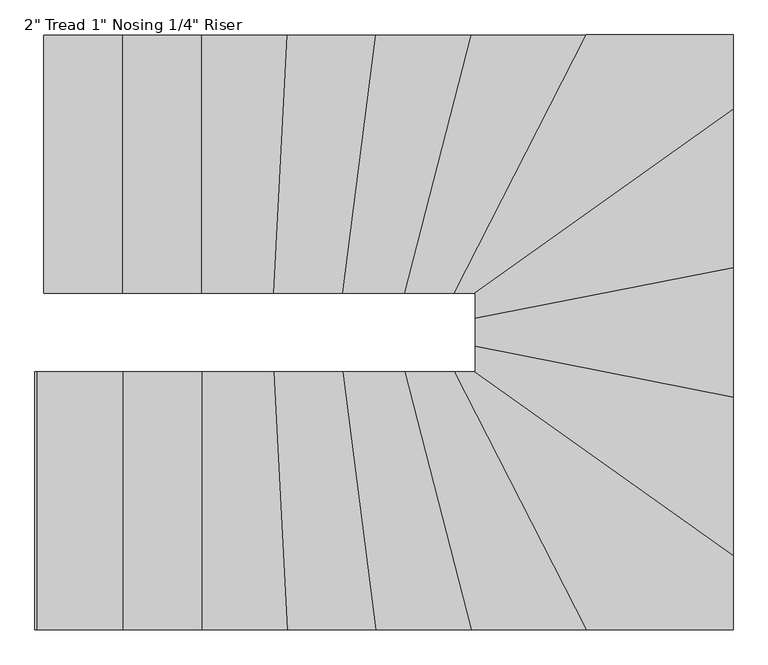
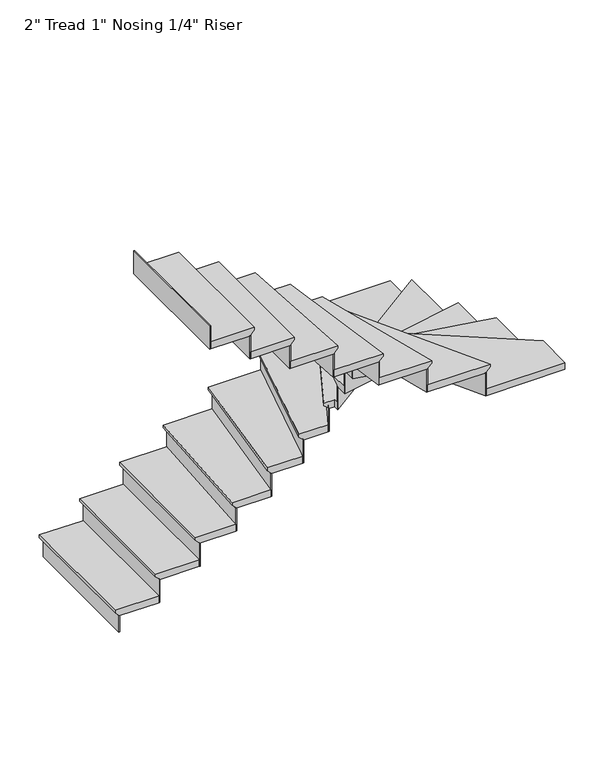
"""IFC4 building model written with IfcOpenShell, lengths in millimetres: stair flight geometry."""

from ifc_helpers import new_model, si_unit, origin, place, context, project, spatial, faceted_brep, source, transform, mapped, element, save


def stair_flight_cc2d1c0a(model_context):
    return source(origin(), model_context, "Body", "Brep", [
        faceted_brep([(3860.8061326, -3914.8192867, 150.2833333), (3860.8061326, -3914.8192867, 169.3333333), (3860.8061326, -3000.4192867, 169.3333333), (3860.8061326, -3000.4192867, 150.2833333), (3886.2061326, -3914.8192867, 124.8833333), (3886.2061326, -3000.4192867, 124.8833333), (4165.6061326, -3914.8192867, 169.3333333), (4165.6061326, -3000.4192867, 169.3333333), (3886.2061326, -3000.4192867, 118.5333333), (4165.6061326, -3000.4192867, 118.5333333), (4165.6061326, -3914.8192867, 118.5333333), (3886.2061326, -3914.8192867, 118.5333333)], [[[0, 1, 2, 3]], [[4, 0, 3, 5]], [[2, 1, 6, 7]], [[8, 9, 10, 11]], [[2, 7, 9, 8, 5, 3]], [[8, 11, 4, 5]], [[6, 1, 0, 4, 11, 10]], [[7, 6, 10, 9]]]),
        faceted_brep([(3886.2061326, -3914.8192867, 118.5333333), (3886.2061326, -3914.8192867, 0.0), (3892.5561326, -3914.8192867, 0.0), (3892.5561326, -3914.8192867, 118.5333333), (3886.2061326, -3000.4192867, 118.5333333), (3892.5561326, -3000.4192867, 118.5333333), (3892.5561326, -3000.4192867, 0.0), (3886.2061326, -3000.4192867, 0.0)], [[[0, 1, 2, 3]], [[4, 5, 6, 7]], [[1, 0, 4, 7]], [[2, 1, 7, 6]], [[3, 2, 6, 5]], [[0, 3, 5, 4]]]),
        faceted_brep([(4165.6061326, -3914.8192867, 287.8666667), (4165.6061326, -3914.8192867, 118.5333333), (4171.9561326, -3914.8192867, 118.5333333), (4171.9561326, -3914.8192867, 287.8666667), (4165.6061326, -3000.4192867, 287.8666667), (4171.9561326, -3000.4192867, 287.8666667), (4171.9561326, -3000.4192867, 118.5333333), (4165.6061326, -3000.4192867, 118.5333333)], [[[0, 1, 2, 3]], [[4, 5, 6, 7]], [[1, 0, 4, 7]], [[2, 1, 7, 6]], [[3, 2, 6, 5]], [[0, 3, 5, 4]]]),
        faceted_brep([(4140.2061326, -3000.4192867, 338.6666667), (4140.2061326, -3914.8192867, 338.6666667), (4445.0061326, -3914.8192867, 338.6666667), (4445.0061326, -3000.4192867, 338.6666667), (4165.6061326, -3000.4192867, 287.8666667), (4445.0061326, -3000.4192867, 287.8666667), (4445.0061326, -3914.8192867, 287.8666667), (4165.6061326, -3914.8192867, 287.8666667), (4165.6061326, -3000.4192867, 294.2166667), (4140.2061326, -3000.4192867, 319.6166667), (4165.6061326, -3914.8192867, 294.2166667), (4140.2061326, -3914.8192867, 319.6166667)], [[[0, 1, 2, 3]], [[4, 5, 6, 7]], [[0, 3, 5, 4, 8, 9]], [[4, 7, 10, 8]], [[2, 1, 11, 10, 7, 6]], [[3, 2, 6, 5]], [[11, 1, 0, 9]], [[10, 11, 9, 8]]]),
        faceted_brep([(4445.0061326, -3914.8192867, 457.2), (4445.0061326, -3914.8192867, 287.8666667), (4451.3561326, -3914.8192867, 287.8666667), (4451.3561326, -3914.8192867, 457.2), (4445.0061326, -3000.4192867, 457.2), (4451.3561326, -3000.4192867, 457.2), (4451.3561326, -3000.4192867, 287.8666667), (4445.0061326, -3000.4192867, 287.8666667)], [[[0, 1, 2, 3]], [[4, 5, 6, 7]], [[1, 0, 4, 7]], [[2, 1, 7, 6]], [[3, 2, 6, 5]], [[0, 3, 5, 4]]]),
        faceted_brep([(4419.6061326, -3000.4192867, 508.0), (4419.6061326, -3914.8192867, 508.0), (4700.6732941, -3914.8192867, 508.0), (4748.2075645, -3000.4192867, 508.0), (4445.0061326, -3000.4192867, 457.2), (4748.2075645, -3000.4192867, 457.2), (4700.6732941, -3914.8192867, 457.2), (4445.0061326, -3914.8192867, 457.2), (4445.0061326, -3000.4192867, 463.55), (4419.6061326, -3000.4192867, 488.95), (4445.0061326, -3914.8192867, 463.55), (4419.6061326, -3914.8192867, 488.95)], [[[0, 1, 2, 3]], [[4, 5, 6, 7]], [[0, 3, 5, 4, 8, 9]], [[4, 7, 10, 8]], [[2, 1, 11, 10, 7, 6]], [[3, 2, 6, 5]], [[11, 1, 0, 9]], [[10, 11, 9, 8]]]),
        faceted_brep([(4700.6732941, -3914.8192867, 626.5333333), (4700.6732941, -3914.8192867, 457.2), (4707.0318682, -3914.8192867, 457.2), (4707.0318682, -3914.8192867, 626.5333333), (4748.2075645, -3000.4192867, 626.5333333), (4754.5661386, -3000.4192867, 626.5333333), (4754.5661386, -3000.4192867, 457.2), (4748.2075645, -3000.4192867, 457.2)], [[[0, 1, 2, 3]], [[4, 5, 6, 7]], [[1, 0, 4, 7]], [[2, 1, 7, 6]], [[3, 2, 6, 5]], [[0, 3, 5, 4]]]),
        faceted_brep([(4722.7732678, -3000.4192867, 677.3333333), (4675.2389974, -3914.8192867, 677.3333333), (4944.8399939, -3914.8192867, 677.3333333), (5063.1960455, -3000.4192867, 677.3333333), (4748.2075645, -3000.4192867, 626.5333333), (5063.1960455, -3000.4192867, 626.5333333), (4944.8399939, -3914.8192867, 626.5333333), (4700.6732941, -3914.8192867, 626.5333333), (4748.2075645, -3000.4192867, 632.8833333), (4722.7732678, -3000.4192867, 658.2833333), (4700.6732941, -3914.8192867, 632.8833333), (4675.2389974, -3914.8192867, 658.2833333)], [[[0, 1, 2, 3]], [[4, 5, 6, 7]], [[0, 3, 5, 4, 8, 9]], [[4, 7, 10, 8]], [[2, 1, 11, 10, 7, 6]], [[3, 2, 6, 5]], [[11, 1, 0, 9]], [[10, 11, 9, 8]]]),
        faceted_brep([(4944.8399939, -3914.8192867, 795.8666667), (4944.8399939, -3914.8192867, 626.5333333), (4951.2429657, -3914.8192867, 626.5333333), (4951.2429657, -3914.8192867, 795.8666667), (5063.1960455, -3000.4192867, 795.8666667), (5069.5990173, -3000.4192867, 795.8666667), (5069.5990173, -3000.4192867, 626.5333333), (5063.1960455, -3000.4192867, 626.5333333)], [[[0, 1, 2, 3]], [[4, 5, 6, 7]], [[1, 0, 4, 7]], [[2, 1, 7, 6]], [[3, 2, 6, 5]], [[0, 3, 5, 4]]]),
        faceted_brep([(5037.5841584, -3000.4192867, 846.6666667), (4919.2281068, -3914.8192867, 846.6666667), (5166.4672164, -3914.8192867, 846.6666667), (5401.5976638, -3000.4192867, 846.6666667), (5063.1960455, -3000.4192867, 795.8666667), (5401.5976638, -3000.4192867, 795.8666667), (5166.4672164, -3914.8192867, 795.8666667), (4944.8399939, -3914.8192867, 795.8666667), (5063.1960455, -3000.4192867, 802.2166667), (5037.5841584, -3000.4192867, 827.6166667), (4944.8399939, -3914.8192867, 802.2166667), (4919.2281068, -3914.8192867, 827.6166667)], [[[0, 1, 2, 3]], [[4, 5, 6, 7]], [[0, 3, 5, 4, 8, 9]], [[4, 7, 10, 8]], [[2, 1, 11, 10, 7, 6]], [[3, 2, 6, 5]], [[11, 1, 0, 9]], [[10, 11, 9, 8]]]),
        faceted_brep([(5166.4672164, -3914.8192867, 965.2), (5166.4672164, -3914.8192867, 795.8666667), (5173.0237932, -3914.8192867, 795.8666667), (5173.0237932, -3914.8192867, 965.2), (5401.5976638, -3000.4192867, 965.2), (5408.1542406, -3000.4192867, 965.2), (5408.1542406, -3000.4192867, 795.8666667), (5401.5976638, -3000.4192867, 795.8666667)], [[[0, 1, 2, 3]], [[4, 5, 6, 7]], [[1, 0, 4, 7]], [[2, 1, 7, 6]], [[3, 2, 6, 5]], [[0, 3, 5, 4]]]),
        faceted_brep([(5375.3713563, -3000.4192867, 1016.0), (5140.2409089, -3914.8192867, 1016.0), (5342.8138524, -3914.8192867, 1016.0), (5811.6384738, -3000.4192867, 1016.0), (5401.5976638, -3000.4192867, 965.2), (5811.6384738, -3000.4192867, 965.2), (5342.8138524, -3914.8192867, 965.2), (5166.4672164, -3914.8192867, 965.2), (5401.5976638, -3000.4192867, 971.55), (5375.3713563, -3000.4192867, 996.95), (5166.4672164, -3914.8192867, 971.55), (5140.2409089, -3914.8192867, 996.95)], [[[0, 1, 2, 3]], [[4, 5, 6, 7]], [[0, 3, 5, 4, 8, 9]], [[4, 7, 10, 8]], [[2, 1, 11, 10, 7, 6]], [[3, 2, 6, 5]], [[11, 1, 0, 9]], [[10, 11, 9, 8]]]),
        faceted_brep([(5342.8138524, -3914.8192867, 1134.5333333), (5342.8138524, -3914.8192867, 965.2), (5349.9498356, -3914.8192867, 965.2), (5349.9498356, -3914.8192867, 1134.5333333), (5811.6384738, -3000.4192867, 1134.5333333), (5818.7744569, -3000.4192867, 1134.5333333), (5818.7744569, -3000.4192867, 965.2), (5811.6384738, -3000.4192867, 965.2)], [[[0, 1, 2, 3]], [[4, 5, 6, 7]], [[1, 0, 4, 7]], [[2, 1, 7, 6]], [[3, 2, 6, 5]], [[0, 3, 5, 4]]]),
        faceted_brep([(6302.9378245, -3294.1004204, 1185.3333333), (6302.9378245, -3000.4192867, 1185.3333333), (5783.0945412, -3000.4192867, 1185.3333333), (5314.2699199, -3914.8192867, 1185.3333333), (5388.5378245, -3914.8192867, 1185.3333333), (5388.5378245, -3944.3743695, 1185.3333333), (6302.9378245, -3000.4192867, 1134.5333333), (6302.9378245, -3294.1004204, 1134.5333333), (5388.5378245, -3944.3743695, 1134.5333333), (5388.5378245, -3914.8192867, 1134.5333333), (5342.8138524, -3914.8192867, 1134.5333333), (5811.6384738, -3000.4192867, 1134.5333333), (5811.6384738, -3000.4192867, 1140.8833333), (5783.0945412, -3000.4192867, 1166.2833333), (5342.8138524, -3914.8192867, 1140.8833333), (5314.2699199, -3914.8192867, 1166.2833333)], [[[0, 1, 2, 3, 4, 5]], [[6, 7, 8, 9, 10, 11]], [[1, 0, 7, 6]], [[2, 1, 6, 11, 12, 13]], [[11, 10, 14, 12]], [[4, 3, 15, 14, 10, 9]], [[5, 4, 9, 8]], [[0, 5, 8, 7]], [[15, 3, 2, 13]], [[14, 15, 13, 12]]]),
        faceted_brep([(5388.5378245, -3944.3743695, 1303.8666667), (5388.5378245, -3944.3743695, 1134.5333333), (5388.5378245, -3952.1663443, 1134.5333333), (5388.5378245, -3952.1663443, 1303.8666667), (6302.9378245, -3294.1004204, 1303.8666667), (6302.9378245, -3301.8923952, 1303.8666667), (6302.9378245, -3301.8923952, 1134.5333333), (6302.9378245, -3294.1004204, 1134.5333333)], [[[0, 1, 2, 3]], [[4, 5, 6, 7]], [[1, 0, 4, 7]], [[2, 1, 7, 6]], [[3, 2, 6, 5]], [[0, 3, 5, 4]]]),
        faceted_brep([(6302.9378245, -3262.9325212, 1354.6666667), (5388.5378245, -3913.2064704, 1354.6666667), (5388.5378245, -4030.8284566, 1354.6666667), (6302.9378245, -3850.5876003, 1354.6666667), (6302.9378245, -3294.1004204, 1303.8666667), (6302.9378245, -3850.5876003, 1303.8666667), (5388.5378245, -4030.8284566, 1303.8666667), (5388.5378245, -3944.3743695, 1303.8666667), (6302.9378245, -3294.1004204, 1310.2166667), (6302.9378245, -3262.9325212, 1335.6166667), (5388.5378245, -3944.3743695, 1310.2166667), (5388.5378245, -3913.2064704, 1335.6166667)], [[[0, 1, 2, 3]], [[4, 5, 6, 7]], [[0, 3, 5, 4, 8, 9]], [[4, 7, 10, 8]], [[2, 1, 11, 10, 7, 6]], [[3, 2, 6, 5]], [[11, 1, 0, 9]], [[10, 11, 9, 8]]]),
        faceted_brep([(5388.5378245, -4030.8284566, 1473.2), (5388.5378245, -4030.8284566, 1303.8666667), (5388.5378245, -4037.300642, 1303.8666667), (5388.5378245, -4037.300642, 1473.2), (6302.9378245, -3850.5876003, 1473.2), (6302.9378245, -3857.0597857, 1473.2), (6302.9378245, -3857.0597857, 1303.8666667), (6302.9378245, -3850.5876003, 1303.8666667)], [[[0, 1, 2, 3]], [[4, 5, 6, 7]], [[1, 0, 4, 7]], [[2, 1, 7, 6]], [[3, 2, 6, 5]], [[0, 3, 5, 4]]]),
        faceted_brep([(6302.9378245, -3824.6988585, 1524.0), (5388.5378245, -4004.9397148, 1524.0), (5388.5378245, -4129.9876003, 1524.0), (6302.9378245, -4310.2284566, 1524.0), (6302.9378245, -3850.5876003, 1473.2), (6302.9378245, -4310.2284566, 1473.2), (5388.5378245, -4129.9876003, 1473.2), (5388.5378245, -4030.8284566, 1473.2), (6302.9378245, -3850.5876003, 1479.55), (6302.9378245, -3824.6988585, 1504.95), (5388.5378245, -4030.8284566, 1479.55), (5388.5378245, -4004.9397148, 1504.95)], [[[0, 1, 2, 3]], [[4, 5, 6, 7]], [[0, 3, 5, 4, 8, 9]], [[4, 7, 10, 8]], [[2, 1, 11, 10, 7, 6]], [[3, 2, 6, 5]], [[11, 1, 0, 9]], [[10, 11, 9, 8]]]),
        faceted_brep([(5388.5378245, -4129.9876003, 1642.5333333), (5388.5378245, -4129.9876003, 1473.2), (5388.5378245, -4136.4597857, 1473.2), (5388.5378245, -4136.4597857, 1642.5333333), (6302.9378245, -4310.2284566, 1642.5333333), (6302.9378245, -4316.700642, 1642.5333333), (6302.9378245, -4316.700642, 1473.2), (6302.9378245, -4310.2284566, 1473.2)], [[[0, 1, 2, 3]], [[4, 5, 6, 7]], [[1, 0, 4, 7]], [[2, 1, 7, 6]], [[3, 2, 6, 5]], [[0, 3, 5, 4]]]),
        faceted_brep([(6302.9378245, -4284.3397148, 1693.3333333), (5388.5378245, -4104.0988585, 1693.3333333), (5388.5378245, -4194.2192867, 1693.3333333), (5342.4423499, -4194.2192867, 1693.3333333), (6302.9378245, -4877.2739513, 1693.3333333), (6302.9378245, -4310.2284566, 1642.5333333), (6302.9378245, -4877.2739513, 1642.5333333), (5342.4423499, -4194.2192867, 1642.5333333), (5388.5378245, -4194.2192867, 1642.5333333), (5388.5378245, -4129.9876003, 1642.5333333), (6302.9378245, -4310.2284566, 1648.8833333), (6302.9378245, -4284.3397148, 1674.2833333), (5388.5378245, -4129.9876003, 1648.8833333), (5388.5378245, -4104.0988585, 1674.2833333)], [[[0, 1, 2, 3, 4]], [[5, 6, 7, 8, 9]], [[0, 4, 6, 5, 10, 11]], [[5, 9, 12, 10]], [[2, 1, 13, 12, 9, 8]], [[3, 2, 8, 7]], [[4, 3, 7, 6]], [[13, 1, 0, 11]], [[12, 13, 11, 10]]]),
        faceted_brep([(5342.4423499, -4194.2192867, 1811.8666667), (5342.4423499, -4194.2192867, 1642.5333333), (5331.4854574, -4194.2192867, 1642.5333333), (5331.4854574, -4194.2192867, 1811.8666667), (6302.9378245, -4877.2739513, 1811.8666667), (6302.9378245, -4885.0659261, 1811.8666667), (6302.9378245, -4885.0659261, 1642.5333333), (6302.9378245, -4877.2739513, 1642.5333333)], [[[0, 1, 2, 3]], [[4, 5, 6, 7]], [[1, 0, 4, 7]], [[2, 1, 7, 6]], [[3, 2, 6, 5]], [[0, 3, 5, 4]]]),
        faceted_brep([(5754.5506087, -5108.6192867, 1862.6666667), (6302.9378245, -5108.6192867, 1862.6666667), (6302.9378245, -4846.1060522, 1862.6666667), (5386.2699199, -4194.2192867, 1862.6666667), (5285.7259874, -4194.2192867, 1862.6666667), (6302.9378245, -5108.6192867, 1811.8666667), (5754.5506087, -5108.6192867, 1811.8666667), (5285.7259874, -4194.2192867, 1811.8666667), (5342.4423499, -4194.2192867, 1811.8666667), (6302.9378245, -4877.2739513, 1811.8666667), (6302.9378245, -4877.2739513, 1818.2166667), (6302.9378245, -4846.1060522, 1843.6166667), (5342.4423499, -4194.2192867, 1818.2166667), (5386.2699199, -4194.2192867, 1843.6166667)], [[[0, 1, 2, 3, 4]], [[5, 6, 7, 8, 9]], [[1, 0, 6, 5]], [[2, 1, 5, 9, 10, 11]], [[9, 8, 12, 10]], [[4, 3, 13, 12, 8, 7]], [[0, 4, 7, 6]], [[13, 3, 2, 11]], [[12, 13, 11, 10]]]),
        faceted_brep([(5285.7259874, -4194.2192867, 1981.2), (5285.7259874, -4194.2192867, 1811.8666667), (5278.5900042, -4194.2192867, 1811.8666667), (5278.5900042, -4194.2192867, 1981.2), (5754.5506087, -5108.6192867, 1981.2), (5747.4146256, -5108.6192867, 1981.2), (5747.4146256, -5108.6192867, 1811.8666667), (5754.5506087, -5108.6192867, 1811.8666667)], [[[0, 1, 2, 3]], [[4, 5, 6, 7]], [[1, 0, 4, 7]], [[2, 1, 7, 6]], [[3, 2, 6, 5]], [[0, 3, 5, 4]]]),
        faceted_brep([(5783.0945412, -5108.6192867, 2032.0), (5314.2699199, -4194.2192867, 2032.0), (5114.0146014, -4194.2192867, 2032.0), (5349.1450488, -5108.6192867, 2032.0), (5754.5506087, -5108.6192867, 1981.2), (5349.1450488, -5108.6192867, 1981.2), (5114.0146014, -4194.2192867, 1981.2), (5285.7259874, -4194.2192867, 1981.2), (5754.5506087, -5108.6192867, 1987.55), (5783.0945412, -5108.6192867, 2012.95), (5285.7259874, -4194.2192867, 1987.55), (5314.2699199, -4194.2192867, 2012.95)], [[[0, 1, 2, 3]], [[4, 5, 6, 7]], [[0, 3, 5, 4, 8, 9]], [[4, 7, 10, 8]], [[2, 1, 11, 10, 7, 6]], [[3, 2, 6, 5]], [[11, 1, 0, 9]], [[10, 11, 9, 8]]]),
        faceted_brep([(5114.0146014, -4194.2192867, 2150.5333333), (5114.0146014, -4194.2192867, 1981.2), (5107.4580246, -4194.2192867, 1981.2), (5107.4580246, -4194.2192867, 2150.5333333), (5349.1450488, -5108.6192867, 2150.5333333), (5342.588472, -5108.6192867, 2150.5333333), (5342.588472, -5108.6192867, 1981.2), (5349.1450488, -5108.6192867, 1981.2)], [[[0, 1, 2, 3]], [[4, 5, 6, 7]], [[1, 0, 4, 7]], [[2, 1, 7, 6]], [[3, 2, 6, 5]], [[0, 3, 5, 4]]]),
        faceted_brep([(5375.3713563, -5108.6192867, 2201.3333333), (5140.2409089, -4194.2192867, 2201.3333333), (4893.6162196, -4194.2192867, 2201.3333333), (5011.9722713, -5108.6192867, 2201.3333333), (5349.1450488, -5108.6192867, 2150.5333333), (5011.9722713, -5108.6192867, 2150.5333333), (4893.6162196, -4194.2192867, 2150.5333333), (5114.0146014, -4194.2192867, 2150.5333333), (5349.1450488, -5108.6192867, 2156.8833333), (5375.3713563, -5108.6192867, 2182.2833333), (5114.0146014, -4194.2192867, 2156.8833333), (5140.2409089, -4194.2192867, 2182.2833333)], [[[0, 1, 2, 3]], [[4, 5, 6, 7]], [[0, 3, 5, 4, 8, 9]], [[4, 7, 10, 8]], [[2, 1, 11, 10, 7, 6]], [[3, 2, 6, 5]], [[11, 1, 0, 9]], [[10, 11, 9, 8]]]),
        faceted_brep([(4893.6162196, -4194.2192867, 2319.8666667), (4893.6162196, -4194.2192867, 2150.5333333), (4887.2132479, -4194.2192867, 2150.5333333), (4887.2132479, -4194.2192867, 2319.8666667), (5011.9722713, -5108.6192867, 2319.8666667), (5005.5692995, -5108.6192867, 2319.8666667), (5005.5692995, -5108.6192867, 2150.5333333), (5011.9722713, -5108.6192867, 2150.5333333)], [[[0, 1, 2, 3]], [[4, 5, 6, 7]], [[1, 0, 4, 7]], [[2, 1, 7, 6]], [[3, 2, 6, 5]], [[0, 3, 5, 4]]]),
        faceted_brep([(5037.5841584, -5108.6192867, 2370.6666667), (4919.2281068, -4194.2192867, 2370.6666667), (4649.8047007, -4194.2192867, 2370.6666667), (4697.3389711, -5108.6192867, 2370.6666667), (5011.9722713, -5108.6192867, 2319.8666667), (4697.3389711, -5108.6192867, 2319.8666667), (4649.8047007, -4194.2192867, 2319.8666667), (4893.6162196, -4194.2192867, 2319.8666667), (5011.9722713, -5108.6192867, 2326.2166667), (5037.5841584, -5108.6192867, 2351.6166667), (4893.6162196, -4194.2192867, 2326.2166667), (4919.2281068, -4194.2192867, 2351.6166667)], [[[0, 1, 2, 3]], [[4, 5, 6, 7]], [[0, 3, 5, 4, 8, 9]], [[4, 7, 10, 8]], [[2, 1, 11, 10, 7, 6]], [[3, 2, 6, 5]], [[11, 1, 0, 9]], [[10, 11, 9, 8]]]),
        faceted_brep([(4649.8047007, -4194.2192867, 2489.2), (4649.8047007, -4194.2192867, 2319.8666667), (4643.4461266, -4194.2192867, 2319.8666667), (4643.4461266, -4194.2192867, 2489.2), (4697.3389711, -5108.6192867, 2489.2), (4690.980397, -5108.6192867, 2489.2), (4690.980397, -5108.6192867, 2319.8666667), (4697.3389711, -5108.6192867, 2319.8666667)], [[[0, 1, 2, 3]], [[4, 5, 6, 7]], [[1, 0, 4, 7]], [[2, 1, 7, 6]], [[3, 2, 6, 5]], [[0, 3, 5, 4]]]),
        faceted_brep([(4722.7732678, -5108.6192867, 2540.0), (4675.2389974, -4194.2192867, 2540.0), (4394.2061326, -4194.2192867, 2540.0), (4394.2061326, -5108.6192867, 2540.0), (4697.3389711, -5108.6192867, 2489.2), (4394.2061326, -5108.6192867, 2489.2), (4394.2061326, -4194.2192867, 2489.2), (4649.8047007, -4194.2192867, 2489.2), (4697.3389711, -5108.6192867, 2495.55), (4722.7732678, -5108.6192867, 2520.95), (4649.8047007, -4194.2192867, 2495.55), (4675.2389974, -4194.2192867, 2520.95)], [[[0, 1, 2, 3]], [[4, 5, 6, 7]], [[0, 3, 5, 4, 8, 9]], [[4, 7, 10, 8]], [[2, 1, 11, 10, 7, 6]], [[3, 2, 6, 5]], [[11, 1, 0, 9]], [[10, 11, 9, 8]]]),
        faceted_brep([(4394.2061326, -4194.2192867, 2658.5333333), (4394.2061326, -4194.2192867, 2489.2), (4387.8561326, -4194.2192867, 2489.2), (4387.8561326, -4194.2192867, 2658.5333333), (4394.2061326, -5108.6192867, 2658.5333333), (4387.8561326, -5108.6192867, 2658.5333333), (4387.8561326, -5108.6192867, 2489.2), (4394.2061326, -5108.6192867, 2489.2)], [[[0, 1, 2, 3]], [[4, 5, 6, 7]], [[1, 0, 4, 7]], [[2, 1, 7, 6]], [[3, 2, 6, 5]], [[0, 3, 5, 4]]]),
        faceted_brep([(4419.6061326, -5108.6192867, 2709.3333333), (4419.6061326, -4194.2192867, 2709.3333333), (4114.8061326, -4194.2192867, 2709.3333333), (4114.8061326, -5108.6192867, 2709.3333333), (4394.2061326, -5108.6192867, 2658.5333333), (4114.8061326, -5108.6192867, 2658.5333333), (4114.8061326, -4194.2192867, 2658.5333333), (4394.2061326, -4194.2192867, 2658.5333333), (4394.2061326, -5108.6192867, 2664.8833333), (4419.6061326, -5108.6192867, 2690.2833333), (4394.2061326, -4194.2192867, 2664.8833333), (4419.6061326, -4194.2192867, 2690.2833333)], [[[0, 1, 2, 3]], [[4, 5, 6, 7]], [[0, 3, 5, 4, 8, 9]], [[4, 7, 10, 8]], [[2, 1, 11, 10, 7, 6]], [[3, 2, 6, 5]], [[11, 1, 0, 9]], [[10, 11, 9, 8]]]),
        faceted_brep([(4114.8061326, -4194.2192867, 2827.8666667), (4114.8061326, -4194.2192867, 2658.5333333), (4108.4561326, -4194.2192867, 2658.5333333), (4108.4561326, -4194.2192867, 2827.8666667), (4114.8061326, -5108.6192867, 2827.8666667), (4108.4561326, -5108.6192867, 2827.8666667), (4108.4561326, -5108.6192867, 2658.5333333), (4114.8061326, -5108.6192867, 2658.5333333)], [[[0, 1, 2, 3]], [[4, 5, 6, 7]], [[1, 0, 4, 7]], [[2, 1, 7, 6]], [[3, 2, 6, 5]], [[0, 3, 5, 4]]]),
        faceted_brep([(3835.4061326, -4194.2192867, 2997.2), (3835.4061326, -4194.2192867, 2827.8666667), (3829.0561326, -4194.2192867, 2827.8666667), (3829.0561326, -4194.2192867, 2997.2), (3835.4061326, -5108.6192867, 2997.2), (3829.0561326, -5108.6192867, 2997.2), (3829.0561326, -5108.6192867, 2827.8666667), (3835.4061326, -5108.6192867, 2827.8666667)], [[[0, 1, 2, 3]], [[4, 5, 6, 7]], [[1, 0, 4, 7]], [[2, 1, 7, 6]], [[3, 2, 6, 5]], [[0, 3, 5, 4]]]),
        faceted_brep([(4140.2061326, -5108.6192867, 2878.6666667), (4140.2061326, -4194.2192867, 2878.6666667), (3835.4061326, -4194.2192867, 2878.6666667), (3835.4061326, -5108.6192867, 2878.6666667), (4114.8061326, -5108.6192867, 2827.8666667), (3835.4061326, -5108.6192867, 2827.8666667), (3835.4061326, -4194.2192867, 2827.8666667), (4114.8061326, -4194.2192867, 2827.8666667), (4114.8061326, -5108.6192867, 2834.2166667), (4140.2061326, -5108.6192867, 2859.6166667), (4114.8061326, -4194.2192867, 2834.2166667), (4140.2061326, -4194.2192867, 2859.6166667)], [[[0, 1, 2, 3]], [[4, 5, 6, 7]], [[0, 3, 5, 4, 8, 9]], [[4, 7, 10, 8]], [[2, 1, 11, 10, 7, 6]], [[3, 2, 6, 5]], [[11, 1, 0, 9]], [[10, 11, 9, 8]]]),
    ])


if __name__ == "__main__":
    model = new_model("IFC4")
    model_context = context("Model", 3, world=origin())
    ifc_project = project(units=[si_unit("LENGTHUNIT", "METRE", prefix="MILLI")], contexts=[model_context])
    site = spatial("IfcSite", under=ifc_project)
    building = spatial("IfcBuilding", under=site)
    placement = place(None, origin())
    stair_flight_shape = stair_flight_cc2d1c0a(model_context)
    element("IfcStairFlight", 1, ObjectType="2\" Tread 1\" Nosing 1/4\" Riser", at=placement, inside=building, context=model_context, shape_type="MappedRepresentation", body=[
        mapped(stair_flight_shape, transform((0.0, 0.0, 0.0), x_axis=(1.0, 0.0, 0.0), y_axis=(0.0, 1.0, 0.0), z_axis=(0.0, 0.0, 1.0))),
    ])
    save(model, "model.ifc")
